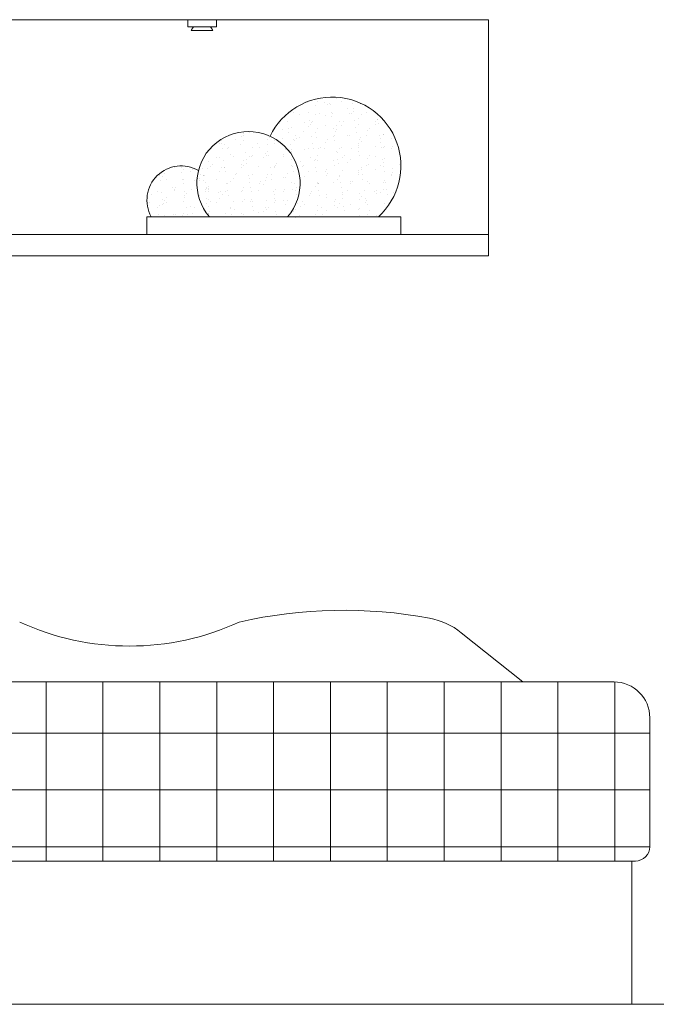
# Model space of a CAD drawing. Units: inches. Extents: x 1994 to 3075, y 3517 to 3950.
# Tile 28 of 58: x 1994.52987 to 1994.56485, y 3553.60329 to 3553.6574. Entities that reach past the tile are written whole.
import ezdxf

# ---------------------------------------------------------------- set-up
doc = ezdxf.new("R2010")
doc.units = ezdxf.units.IN
doc.layers.add('A-FURN-REFR', color=8, linetype='Continuous', lineweight=13)

msp = doc.modelspace()

# ---------------------------------------------------------------- linework, layer by layer
at = {"layer": 'A-FURN-REFR'}
for p, q in [((1994.492639873162, 3553.657398571457), (1994.555631999147, 3553.657398571457)), ((1994.539096566076, 3553.657004870669), (1994.539096566076, 3553.657398571457)), ((1994.539096566076, 3553.657398571457), (1994.540671369225, 3553.657398571457)), ((1994.540671369225, 3553.657004870669), (1994.540671369225, 3553.657398571457)), ((1994.555631999147, 3553.657398571457), (1994.555631999146, 3553.644427213402)), ((1994.539096566075, 3553.657004870669), (1994.540671369225, 3553.657004870669)), ((1994.539293416469, 3553.656808020276), (1994.540474518832, 3553.656808020276)), ((1994.545671567704, 3553.652825872638), (1994.545671567704, 3553.652825872638)), ((1994.546225091408, 3553.652899882358), (1994.546225091408, 3553.652899882358)), ((1994.546596443113, 3553.65285610945), (1994.546596443113, 3553.65285610945)), ((1994.546863187477, 3553.65281113167), (1994.546863187477, 3553.65281113167)), ((1994.547298108168, 3553.653085129387), (1994.547298108168, 3553.653085129387)), ((1994.547521318522, 3553.652886346262), (1994.547521318522, 3553.652886346262)), ((1994.544638888571, 3553.652286427241), (1994.544638888571, 3553.652286427241)), ((1994.544894170837, 3553.652309807435), (1994.544894170837, 3553.652309807435)), ((1994.545023122743, 3553.652512221382), (1994.545023122743, 3553.652512221382)), ((1994.545747841848, 3553.652271457508), (1994.545747841848, 3553.652271457508)), ((1994.546096139502, 3553.652697468411), (1994.546096139502, 3553.652697468411)), ((1994.546782116653, 3553.65272265839), (1994.546782116653, 3553.65272265839)), ((1994.546932370226, 3553.652714015634), (1994.546932370226, 3553.652714015634)), ((1994.546983745335, 3553.652323782936), (1994.546983745335, 3553.652323782936)), ((1994.547894002875, 3553.652521444812), (1994.547894002875, 3553.652521444812)), ((1994.547996152437, 3553.652267530656), (1994.547996152437, 3553.652267530656)), ((1994.548104907986, 3553.65226353994), (1994.548104907986, 3553.65226353994)), ((1994.548168273713, 3553.652766341061), (1994.548168273713, 3553.652766341061)), ((1994.548185978811, 3553.652352013221), (1994.548185978811, 3553.652352013221)), ((1994.548201166313, 3553.652516496956), (1994.548201166313, 3553.652516496956)), ((1994.548568633105, 3553.652769607105), (1994.548568633105, 3553.652769607105)), ((1994.548921027846, 3553.652297767468), (1994.548921027846, 3553.652297767468)), ((1994.544120035292, 3553.651720198246), (1994.544120035292, 3553.651720198246)), ((1994.544557817746, 3553.65219795396), (1994.544557817746, 3553.65219795396)), ((1994.544563313471, 3553.651828899384), (1994.544563313471, 3553.651828899384)), ((1994.54522152621, 3553.65217682022), (1994.54522152621, 3553.65217682022)), ((1994.545490065544, 3553.65174612286), (1994.545490065544, 3553.65174612286)), ((1994.545799216958, 3553.651881224811), (1994.545799216958, 3553.651881224811)), ((1994.54588060908, 3553.651738835511), (1994.54588060908, 3553.651738835511)), ((1994.545961679904, 3553.651827308792), (1994.545961679904, 3553.651827308792)), ((1994.546146401619, 3553.652207057032), (1994.546146401619, 3553.652207057032)), ((1994.546344334198, 3553.652244902675), (1994.546344334198, 3553.652244902675)), ((1994.546692034209, 3553.652133783835), (1994.546692034209, 3553.652133783835)), ((1994.547016637936, 3553.652073938831), (1994.547016637936, 3553.652073938831)), ((1994.547071277028, 3553.652237293845), (1994.547071277028, 3553.652237293845)), ((1994.547429776013, 3553.651792754602), (1994.547429776013, 3553.651792754602)), ((1994.547667125532, 3553.651785784226), (1994.547667125532, 3553.651785784226)), ((1994.548287000338, 3553.651864522816), (1994.548287000338, 3553.651864522816)), ((1994.548502792772, 3553.651978001632), (1994.548502792772, 3553.651978001632)), ((1994.548631744678, 3553.652180415578), (1994.548631744678, 3553.652180415578)), ((1994.54942769932, 3553.651804421491), (1994.54942769932, 3553.651804421491)), ((1994.549508770145, 3553.651892894772), (1994.549508770145, 3553.651892894772)), ((1994.549522903825, 3553.651916848242), (1994.549522903825, 3553.651916848242)), ((1994.542470918336, 3553.651200992831), (1994.542470918336, 3553.651200992831)), ((1994.544288096879, 3553.651358461884), (1994.544288096879, 3553.651358461884)), ((1994.544614688581, 3553.651438666687), (1994.544614688581, 3553.651438666687)), ((1994.544647581181, 3553.651188822582), (1994.544647581181, 3553.651188822582)), ((1994.544793400127, 3553.651499207083), (1994.544793400127, 3553.651499207083)), ((1994.545442826625, 3553.651261079797), (1994.545442826625, 3553.651261079797)), ((1994.545718275536, 3553.651529443895), (1994.545718275536, 3553.651529443895)), ((1994.545832109558, 3553.651631380706), (1994.545832109558, 3553.651631380706)), ((1994.546098855442, 3553.65120267968), (1994.546098855442, 3553.65120267968)), ((1994.546227807348, 3553.651405093626), (1994.546227807348, 3553.651405093626)), ((1994.546643150945, 3553.651559680707), (1994.546643150945, 3553.651559680707)), ((1994.54710247196, 3553.651421964691), (1994.54710247196, 3553.651421964691)), ((1994.547203400413, 3553.651279717062), (1994.547203400413, 3553.651279717062)), ((1994.547284471238, 3553.651368190343), (1994.547284471238, 3553.651368190343)), ((1994.547300824107, 3553.651590340655), (1994.547300824107, 3553.651590340655)), ((1994.547568026354, 3553.651589917519), (1994.547568026354, 3553.651589917519)), ((1994.548338375447, 3553.651474290118), (1994.548338375447, 3553.651474290118)), ((1994.548371268047, 3553.651224446013), (1994.548371268047, 3553.651224446013)), ((1994.548492901763, 3553.65162015433), (1994.548492901763, 3553.65162015433)), ((1994.548989916865, 3553.651326665777), (1994.548989916865, 3553.651326665777)), ((1994.54909868748, 3553.651414317057), (1994.54909868748, 3553.651414317057)), ((1994.549417777172, 3553.651650391142), (1994.549417777172, 3553.651650391142)), ((1994.549555796425, 3553.651667004138), (1994.549555796425, 3553.651667004138)), ((1994.540976954478, 3553.650774880818), (1994.540976954478, 3553.650774880818)), ((1994.541741367432, 3553.650819762049), (1994.541741367432, 3553.650819762049)), ((1994.542049971238, 3553.650960127848), (1994.542049971238, 3553.650960127848)), ((1994.542152382975, 3553.651015315854), (1994.542152382975, 3553.651015315854)), ((1994.542178923144, 3553.651162541795), (1994.542178923144, 3553.651162541795)), ((1994.542185275575, 3553.650765471749), (1994.542185275575, 3553.650765471749)), ((1994.54350194122, 3553.650838399314), (1994.54350194122, 3553.650838399314)), ((1994.543583012045, 3553.650926872594), (1994.543583012045, 3553.650926872594)), ((1994.54384783461, 3553.650784104248), (1994.54384783461, 3553.650784104248)), ((1994.544312677056, 3553.650890139674), (1994.544312677056, 3553.650890139674)), ((1994.544896886777, 3553.650815018703), (1994.544896886777, 3553.650815018703)), ((1994.544979101507, 3553.650755012633), (1994.544979101507, 3553.650755012633)), ((1994.545025838682, 3553.65101743265), (1994.545025838682, 3553.65101743265)), ((1994.545060172331, 3553.650843485914), (1994.545060172331, 3553.650843485914)), ((1994.545237552465, 3553.650920376486), (1994.545237552465, 3553.650920376486)), ((1994.545917943582, 3553.650979406566), (1994.545917943582, 3553.650979406566)), ((1994.546162427874, 3553.650950613298), (1994.546162427874, 3553.650950613298)), ((1994.546694750149, 3553.650638995105), (1994.546694750149, 3553.650638995105)), ((1994.546765617959, 3553.650801961348), (1994.546765617959, 3553.650801961348)), ((1994.547087303283, 3553.65098085011), (1994.547087303283, 3553.65098085011)), ((1994.547153847069, 3553.651031731993), (1994.547153847069, 3553.651031731993)), ((1994.547186739669, 3553.650781887887), (1994.547186739669, 3553.650781887887)), ((1994.547896718814, 3553.65102665608), (1994.547896718814, 3553.65102665608)), ((1994.548012178693, 3553.651011086922), (1994.548012178693, 3553.651011086922)), ((1994.548526191747, 3553.650820598612), (1994.548526191747, 3553.650820598612)), ((1994.548607262571, 3553.650909071893), (1994.548607262571, 3553.650909071893)), ((1994.548634460619, 3553.650685626847), (1994.548634460619, 3553.650685626847)), ((1994.548937054102, 3553.651041323733), (1994.548937054102, 3553.651041323733)), ((1994.549641630449, 3553.651015029997), (1994.549641630449, 3553.651015029997)), ((1994.549707477378, 3553.650870873877), (1994.549707477378, 3553.650870873877)), ((1994.549836429284, 3553.651073287823), (1994.549836429284, 3553.651073287823)), ((1994.549861929511, 3553.651071560545), (1994.549861929511, 3553.651071560545)), ((1994.550312708199, 3553.650867547327), (1994.550312708199, 3553.650867547327)), ((1994.540848002572, 3553.650572466871), (1994.540848002572, 3553.650572466871)), ((1994.540967854597, 3553.650572757729), (1994.540967854597, 3553.650572757729)), ((1994.541000747197, 3553.650322913624), (1994.541000747197, 3553.650322913624)), ((1994.541096001432, 3553.650521703602), (1994.541096001432, 3553.650521703602)), ((1994.541277642314, 3553.650313694884), (1994.541277642314, 3553.650313694884)), ((1994.541358713139, 3553.650402168165), (1994.541358713139, 3553.650402168165)), ((1994.542020876841, 3553.650551940413), (1994.542020876841, 3553.650551940413)), ((1994.542271109599, 3553.650113497608), (1994.542271109599, 3553.650113497608)), ((1994.542645865945, 3553.650396443273), (1994.542645865945, 3553.650396443273)), ((1994.54294575225, 3553.650582177225), (1994.54294575225, 3553.650582177225)), ((1994.543064158765, 3553.6503606436), (1994.543064158765, 3553.6503606436)), ((1994.543455637977, 3553.650556055733), (1994.543455637977, 3553.650556055733)), ((1994.543507013086, 3553.650165823036), (1994.543507013086, 3553.650165823036)), ((1994.543870627659, 3553.650612414037), (1994.543870627659, 3553.650612414037)), ((1994.544456624509, 3553.650240661069), (1994.544456624509, 3553.650240661069)), ((1994.544733415205, 3553.650536848441), (1994.544733415205, 3553.650536848441)), ((1994.544784790315, 3553.650146615743), (1994.544784790315, 3553.650146615743)), ((1994.544787510971, 3553.650271324068), (1994.544787510971, 3553.650271324068)), ((1994.545492781483, 3553.650251334128), (1994.545492781483, 3553.650251334128)), ((1994.54571238638, 3553.65030156088), (1994.54571238638, 3553.65030156088)), ((1994.545969318692, 3553.650589173868), (1994.545969318692, 3553.650589173868)), ((1994.546002211292, 3553.650339329763), (1994.546002211292, 3553.650339329763)), ((1994.54630189284, 3553.650295894184), (1994.54630189284, 3553.650295894184)), ((1994.546382963665, 3553.650384367465), (1994.546382963665, 3553.650384367465)), ((1994.546637261789, 3553.650331797692), (1994.546637261789, 3553.650331797692)), ((1994.547272573694, 3553.650129913747), (1994.547272573694, 3553.650129913747)), ((1994.547303540047, 3553.650095551924), (1994.547303540047, 3553.650095551924)), ((1994.547432491953, 3553.650297965871), (1994.547432491953, 3553.650297965871)), ((1994.547562137198, 3553.650362034504), (1994.547562137198, 3553.650362034504)), ((1994.548088409292, 3553.650342842899), (1994.548088409292, 3553.650342842899)), ((1994.548457102071, 3553.650572471872), (1994.548457102071, 3553.650572471872)), ((1994.548487012608, 3553.650392271316), (1994.548487012608, 3553.650392271316)), ((1994.548505508712, 3553.650483212901), (1994.548505508712, 3553.650483212901)), ((1994.548508477181, 3553.650182239174), (1994.548508477181, 3553.650182239174)), ((1994.549411888016, 3553.650422508127), (1994.549411888016, 3553.650422508127)), ((1994.549693005558, 3553.650624797299), (1994.549693005558, 3553.650624797299)), ((1994.549725898159, 3553.650374953194), (1994.549725898159, 3553.650374953194)), ((1994.54984898308, 3553.650361480163), (1994.54984898308, 3553.650361480163)), ((1994.549930053905, 3553.650449953444), (1994.549930053905, 3553.650449953444)), ((1994.550303372085, 3553.650307189301), (1994.550303372085, 3553.650307189301)), ((1994.550336763426, 3553.650452744939), (1994.550336763426, 3553.650452744939)), ((1994.540241928614, 3553.649621121321), (1994.540241928614, 3553.649621121321)), ((1994.540667875348, 3553.649844090464), (1994.540667875348, 3553.649844090464)), ((1994.540839859859, 3553.649835939171), (1994.540839859859, 3553.649835939171)), ((1994.541086581222, 3553.649670939484), (1994.541086581222, 3553.649670939484)), ((1994.541443897279, 3553.650008782297), (1994.541443897279, 3553.650008782297)), ((1994.541592750758, 3553.649874327276), (1994.541592750758, 3553.649874327276)), ((1994.542181639084, 3553.649667753064), (1994.542181639084, 3553.649667753064)), ((1994.542322484709, 3553.649723264911), (1994.542322484709, 3553.649723264911)), ((1994.542517626167, 3553.649904564088), (1994.542517626167, 3553.649904564088)), ((1994.542600433647, 3553.649854576435), (1994.542600433647, 3553.649854576435)), ((1994.542681504472, 3553.649943049716), (1994.542681504472, 3553.649943049716)), ((1994.543254655843, 3553.649853000092), (1994.543254655843, 3553.649853000092)), ((1994.543383607749, 3553.650055414039), (1994.543383607749, 3553.650055414039)), ((1994.543442501576, 3553.6499348009), (1994.543442501576, 3553.6499348009)), ((1994.543539905686, 3553.649915978931), (1994.543539905686, 3553.649915978931)), ((1994.544367376985, 3553.649965037712), (1994.544367376985, 3553.649965037712)), ((1994.544386950099, 3553.64990152515), (1994.544386950099, 3553.64990152515)), ((1994.544810268088, 3553.649706562914), (1994.544810268088, 3553.649706562914)), ((1994.545284260297, 3553.649623947742), (1994.545284260297, 3553.649623947742)), ((1994.545864110386, 3553.649818138469), (1994.545864110386, 3553.649818138469)), ((1994.546088045316, 3553.649687355623), (1994.546088045316, 3553.649687355623)), ((1994.546101571382, 3553.649707890949), (1994.546101571382, 3553.649707890949)), ((1994.546209135706, 3553.649654184555), (1994.546209135706, 3553.649654184555)), ((1994.546230523287, 3553.649910304895), (1994.546230523287, 3553.649910304895)), ((1994.547134011115, 3553.649684421367), (1994.547134011115, 3553.649684421367)), ((1994.547323948803, 3553.64973968105), (1994.547323948803, 3553.64973968105)), ((1994.547624684173, 3553.649836775735), (1994.547624684173, 3553.649836775735)), ((1994.547705754999, 3553.649925249015), (1994.547705754999, 3553.649925249015)), ((1994.548058886525, 3553.649714658178), (1994.548058886525, 3553.649714658178)), ((1994.548541369781, 3553.64993239507), (1994.548541369781, 3553.64993239507)), ((1994.548983761933, 3553.64974489499), (1994.548983761933, 3553.64974489499)), ((1994.54910140342, 3553.649919528325), (1994.54910140342, 3553.649919528325)), ((1994.549411200625, 3553.649883724449), (1994.549411200625, 3553.649883724449)), ((1994.549811732183, 3553.649722979054), (1994.549811732183, 3553.649722979054)), ((1994.549839145223, 3553.649578499092), (1994.549839145223, 3553.649578499092)), ((1994.549908637343, 3553.649775131802), (1994.549908637343, 3553.649775131802)), ((1994.538349954585, 3553.649268434922), (1994.538349954585, 3553.649268434922)), ((1994.53874159335, 3553.649274475566), (1994.53874159335, 3553.649274475566)), ((1994.538774485951, 3553.649024631461), (1994.538774485951, 3553.649024631461)), ((1994.538893768846, 3553.649147539603), (1994.538893768846, 3553.649147539603)), ((1994.539267433067, 3553.649068890523), (1994.539267433067, 3553.649068890523)), ((1994.539348503892, 3553.649157363803), (1994.539348503892, 3553.649157363803)), ((1994.539902052844, 3553.649228381359), (1994.539902052844, 3553.649228381359)), ((1994.540187152278, 3553.649235023055), (1994.540187152278, 3553.649235023055)), ((1994.540376134741, 3553.649329872007), (1994.540376134741, 3553.649329872007)), ((1994.540457205566, 3553.649418345287), (1994.540457205566, 3553.649418345287)), ((1994.540850718512, 3553.649077678141), (1994.540850718512, 3553.649077678141)), ((1994.540979670418, 3553.649280092088), (1994.540979670418, 3553.649280092088)), ((1994.541112027687, 3553.649265259867), (1994.541112027687, 3553.649265259867)), ((1994.541137956331, 3553.649280706786), (1994.541137956331, 3553.649280706786)), ((1994.541170848932, 3553.649030862681), (1994.541170848932, 3553.649030862681)), ((1994.542036903096, 3553.649295496679), (1994.542036903096, 3553.649295496679)), ((1994.542052687177, 3553.649465339117), (1994.542052687177, 3553.649465339117)), ((1994.542162651192, 3553.649376820721), (1994.542162651192, 3553.649376820721)), ((1994.542355377309, 3553.649473420806), (1994.542355377309, 3553.649473420806)), ((1994.542961778506, 3553.64932573349), (1994.542961778506, 3553.64932573349)), ((1994.543625739711, 3553.64926400479), (1994.543625739711, 3553.64926400479)), ((1994.54385055055, 3553.649289315518), (1994.54385055055, 3553.649289315518)), ((1994.543886653915, 3553.649355970303), (1994.543886653915, 3553.649355970303)), ((1994.543923224981, 3553.649395457986), (1994.543923224981, 3553.649395457986)), ((1994.544004295805, 3553.649483931267), (1994.544004295805, 3553.649483931267)), ((1994.544811529324, 3553.649386207115), (1994.544811529324, 3553.649386207115)), ((1994.544861643197, 3553.649316330217), (1994.544861643197, 3553.649316330217)), ((1994.544894535798, 3553.649066486112), (1994.544894535798, 3553.649066486112)), ((1994.545400385267, 3553.649312071306), (1994.545400385267, 3553.649312071306)), ((1994.545481456092, 3553.649400544586), (1994.545481456092, 3553.649400544586)), ((1994.545728412635, 3553.649045117146), (1994.545728412635, 3553.649045117146)), ((1994.546139420425, 3553.649297122924), (1994.546139420425, 3553.649297122924)), ((1994.546172313026, 3553.64904727882), (1994.546172313026, 3553.64904727882)), ((1994.546653288045, 3553.649075353957), (1994.546653288045, 3553.649075353957)), ((1994.546697466088, 3553.649144206373), (1994.546697466088, 3553.649144206373)), ((1994.547186901719, 3553.64935902002), (1994.547186901719, 3553.64935902002)), ((1994.547356841404, 3553.649489836944), (1994.547356841404, 3553.649489836944)), ((1994.547578163454, 3553.649105590769), (1994.547578163454, 3553.649105590769)), ((1994.547899434754, 3553.64953186735), (1994.547899434754, 3553.64953186735)), ((1994.548503038863, 3553.649135827581), (1994.548503038863, 3553.649135827581)), ((1994.548627203805, 3553.649280420928), (1994.548627203805, 3553.649280420928)), ((1994.548637176558, 3553.649190838116), (1994.548637176558, 3553.649190838116)), ((1994.548947475507, 3553.649377657285), (1994.548947475507, 3553.649377657285)), ((1994.549028546332, 3553.649466130565), (1994.549028546332, 3553.649466130565)), ((1994.549427914272, 3553.649166064393), (1994.549427914272, 3553.649166064393)), ((1994.549710193317, 3553.649376085144), (1994.549710193317, 3553.649376085144)), ((1994.549863107292, 3553.649332746356), (1994.549863107292, 3553.649332746356)), ((1994.549895999892, 3553.649082902251), (1994.549895999892, 3553.649082902251)), ((1994.550351337665, 3553.649007012116), (1994.550351337665, 3553.649007012116)), ((1994.550352789681, 3553.649196301205), (1994.550352789681, 3553.649196301205)), ((1994.550733991959, 3553.649424606), (1994.550733991959, 3553.649424606)), ((1994.537557064973, 3553.648831917442), (1994.537557064973, 3553.648831917442)), ((1994.537589957573, 3553.648582073337), (1994.537589957573, 3553.648582073337)), ((1994.537691800181, 3553.648759878627), (1994.537691800181, 3553.648759878627)), ((1994.537820752087, 3553.648962292573), (1994.537820752087, 3553.648962292573)), ((1994.537921828502, 3553.648590821784), (1994.537921828502, 3553.648590821784)), ((1994.538829650613, 3553.648591134808), (1994.538829650613, 3553.648591134808)), ((1994.538846703912, 3553.648621058596), (1994.538846703912, 3553.648621058596)), ((1994.539489663553, 3553.648583855028), (1994.539489663553, 3553.648583855028)), ((1994.539648749847, 3553.648690017165), (1994.539648749847, 3553.648690017165)), ((1994.539737110784, 3553.648585970638), (1994.539737110784, 3553.648585970638)), ((1994.53977157932, 3553.648651295408), (1994.53977157932, 3553.648651295408)), ((1994.539777701752, 3553.648892431112), (1994.539777701752, 3553.648892431112)), ((1994.539938352286, 3553.648852116292), (1994.539938352286, 3553.648852116292)), ((1994.539953427954, 3553.648838148661), (1994.539953427954, 3553.648838148661)), ((1994.539986320554, 3553.648588304556), (1994.539986320554, 3553.648588304556)), ((1994.540044848352, 3553.648815215446), (1994.540044848352, 3553.648815215446)), ((1994.540661986192, 3553.64861620745), (1994.540661986192, 3553.64861620745)), ((1994.541446613219, 3553.648513993566), (1994.541446613219, 3553.648513993566)), ((1994.541586861602, 3553.648646444262), (1994.541586861602, 3553.648646444262)), ((1994.541698926074, 3553.648870753558), (1994.541698926074, 3553.648870753558)), ((1994.541779996899, 3553.648959226837), (1994.541779996899, 3553.648959226837)), ((1994.542441211333, 3553.648821446664), (1994.542441211333, 3553.648821446664)), ((1994.542511737011, 3553.648676681073), (1994.542511737011, 3553.648676681073)), ((1994.542648581884, 3553.648901654541), (1994.542648581884, 3553.648901654541)), ((1994.543102788233, 3553.648500108388), (1994.543102788233, 3553.648500108388)), ((1994.543386323688, 3553.648560625308), (1994.543386323688, 3553.648560625308)), ((1994.54343661242, 3553.648706917885), (1994.54343661242, 3553.648706917885)), ((1994.543485442526, 3553.648917702272), (1994.543485442526, 3553.648917702272)), ((1994.54367711482, 3553.648873772092), (1994.54367711482, 3553.648873772092)), ((1994.54371000742, 3553.648623927987), (1994.54371000742, 3553.648623927987)), ((1994.544361487829, 3553.648737154698), (1994.544361487829, 3553.648737154698)), ((1994.544459340448, 3553.648745872337), (1994.544459340448, 3553.648745872337)), ((1994.544588292354, 3553.648948286284), (1994.544588292354, 3553.648948286284)), ((1994.545495497423, 3553.648756545398), (1994.545495497423, 3553.648756545398)), ((1994.5467231766, 3553.648852952856), (1994.5467231766, 3553.648852952856)), ((1994.546804247425, 3553.648941426137), (1994.546804247425, 3553.648941426137)), ((1994.547306255986, 3553.648600763193), (1994.547306255986, 3553.648600763193)), ((1994.547435207893, 3553.64880317714), (1994.547435207893, 3553.64880317714)), ((1994.547442675427, 3553.648837862804), (1994.547442675427, 3553.648837862804)), ((1994.548052997368, 3553.648486775164), (1994.548052997368, 3553.648486775164)), ((1994.548127038759, 3553.648482307687), (1994.548127038759, 3553.648482307687)), ((1994.548508224652, 3553.648988424169), (1994.548508224652, 3553.648988424169)), ((1994.548509693052, 3553.648899901571), (1994.548509693052, 3553.648899901571)), ((1994.548678578915, 3553.648890188231), (1994.548678578915, 3553.648890188231)), ((1994.548711471515, 3553.648640344126), (1994.548711471515, 3553.648640344126)), ((1994.548977872777, 3553.648517011976), (1994.548977872777, 3553.648517011976)), ((1994.549902748187, 3553.648547248787), (1994.549902748187, 3553.648547248787)), ((1994.55027026684, 3553.648918538836), (1994.55027026684, 3553.648918538836)), ((1994.550306088024, 3553.648812400569), (1994.550306088024, 3553.648812400569)), ((1994.537441105432, 3553.647981754375), (1994.537441105432, 3553.647981754375)), ((1994.537675791597, 3553.647930099196), (1994.537675791597, 3553.647930099196)), ((1994.538287694888, 3553.648196194052), (1994.538287694888, 3553.648196194052)), ((1994.538365925494, 3553.648085067644), (1994.538365925494, 3553.648085067644)), ((1994.538365980841, 3553.648011991187), (1994.538365980841, 3553.648011991187)), ((1994.538446996319, 3553.648173540925), (1994.538446996319, 3553.648173540925)), ((1994.538860319974, 3553.64837265732), (1994.538860319974, 3553.64837265732)), ((1994.538911695084, 3553.647982424623), (1994.538911695084, 3553.647982424623)), ((1994.53929085625, 3553.648042227999), (1994.53929085625, 3553.648042227999)), ((1994.540072154578, 3553.647936330416), (1994.540072154578, 3553.647936330416)), ((1994.540096223462, 3553.648424982748), (1994.540096223462, 3553.648424982748)), ((1994.540098453451, 3553.648040411848), (1994.540098453451, 3553.648040411848)), ((1994.540129116062, 3553.648175138643), (1994.540129116062, 3553.648175138643)), ((1994.540152441946, 3553.648132016359), (1994.540152441946, 3553.648132016359)), ((1994.540215731659, 3553.648072464811), (1994.540215731659, 3553.648072464811)), ((1994.540227405357, 3553.648242825795), (1994.540227405357, 3553.648242825795)), ((1994.54023386011, 3553.647938594312), (1994.54023386011, 3553.647938594312)), ((1994.540244644554, 3553.64812633259), (1994.540244644554, 3553.64812633259)), ((1994.540878489326, 3553.647975403959), (1994.540878489326, 3553.647975403959)), ((1994.541158735519, 3553.647968831124), (1994.541158735519, 3553.647968831124)), ((1994.541256682955, 3553.64837888854), (1994.541256682955, 3553.64837888854)), ((1994.54126114362, 3553.648392997843), (1994.54126114362, 3553.648392997843)), ((1994.541308058065, 3553.647988655843), (1994.541308058065, 3553.647988655843)), ((1994.542055403117, 3553.647970550385), (1994.542055403117, 3553.647970550385)), ((1994.542083610928, 3553.647999067936), (1994.542083610928, 3553.647999067936)), ((1994.542184355023, 3553.648172964332), (1994.542184355023, 3553.648172964332)), ((1994.542492586442, 3553.648431213968), (1994.542492586442, 3553.648431213968)), ((1994.542525479043, 3553.648181369862), (1994.542525479043, 3553.648181369862)), ((1994.542583934953, 3553.647933879393), (1994.542583934953, 3553.647933879393)), ((1994.543008486337, 3553.648029304748), (1994.543008486337, 3553.648029304748)), ((1994.543021717408, 3553.648411635108), (1994.543021717408, 3553.648411635108)), ((1994.543257371782, 3553.648358211361), (1994.543257371782, 3553.648358211361)), ((1994.543795841444, 3553.647971953846), (1994.543795841444, 3553.647971953846)), ((1994.543933361746, 3553.64805954156), (1994.543933361746, 3553.64805954156)), ((1994.544344508742, 3553.647952516659), (1994.544344508742, 3553.647952516659)), ((1994.544425579566, 3553.648040989939), (1994.544425579566, 3553.648040989939)), ((1994.544808233859, 3553.648458583822), (1994.544808233859, 3553.648458583822)), ((1994.544858237155, 3553.648089778371), (1994.544858237155, 3553.648089778371)), ((1994.544980369822, 3553.648414511971), (1994.544980369822, 3553.648414511971)), ((1994.545031744931, 3553.648024279274), (1994.545031744931, 3553.648024279274)), ((1994.545055235155, 3553.648182187763), (1994.545055235155, 3553.648182187763)), ((1994.545278371141, 3553.648396064728), (1994.545278371141, 3553.648396064728)), ((1994.545902739853, 3553.647957603259), (1994.545902739853, 3553.647957603259)), ((1994.546104287321, 3553.648213102217), (1994.546104287321, 3553.648213102217)), ((1994.54620324655, 3553.648426301541), (1994.54620324655, 3553.648426301541)), ((1994.546233239227, 3553.648415516164), (1994.546233239227, 3553.648415516164)), ((1994.54625814705, 3553.648395304679), (1994.54625814705, 3553.648395304679)), ((1994.546285394146, 3553.648375197142), (1994.546285394146, 3553.648375197142)), ((1994.546309522159, 3553.648005071981), (1994.546309522159, 3553.648005071981)), ((1994.547128121959, 3553.648456538352), (1994.547128121959, 3553.648456538352)), ((1994.547494050537, 3553.648447630106), (1994.547494050537, 3553.648447630106)), ((1994.547526943137, 3553.648197786002), (1994.547526943137, 3553.648197786002)), ((1994.547902150694, 3553.648037078618), (1994.547902150694, 3553.648037078618)), ((1994.548045967934, 3553.648393834407), (1994.548045967934, 3553.648393834407)), ((1994.548797305539, 3553.647988369985), (1994.548797305539, 3553.647988369985)), ((1994.549104119359, 3553.648424739594), (1994.549104119359, 3553.648424739594)), ((1994.549368759267, 3553.647934715958), (1994.549368759267, 3553.647934715958)), ((1994.549449830092, 3553.648023189238), (1994.549449830092, 3553.648023189238)), ((1994.549832484386, 3553.648440783122), (1994.549832484386, 3553.648440783122)), ((1994.549841861163, 3553.64808371036), (1994.549841861163, 3553.64808371036)), ((1994.549981833916, 3553.64843092811), (1994.549981833916, 3553.64843092811)), ((1994.550033209026, 3553.648040695413), (1994.550033209026, 3553.648040695413)), ((1994.537085726223, 3553.647808533077), (1994.537085726223, 3553.647808533077)), ((1994.537727166706, 3553.647539866498), (1994.537727166706, 3553.647539866498)), ((1994.537823468026, 3553.647467503843), (1994.537823468026, 3553.647467503843)), ((1994.537928143039, 3553.64760731193), (1994.537928143039, 3553.64760731193)), ((1994.538840814755, 3553.647393175582), (1994.538840814755, 3553.647393175582)), ((1994.538896484786, 3553.647652750872), (1994.538896484786, 3553.647652750872)), ((1994.538944587684, 3553.647732580518), (1994.538944587684, 3553.647732580518)), ((1994.539025436692, 3553.647855164819), (1994.539025436692, 3553.647855164819)), ((1994.539688716827, 3553.647625949195), (1994.539688716827, 3553.647625949195)), ((1994.539765690165, 3553.647423412394), (1994.539765690165, 3553.647423412394)), ((1994.539769787652, 3553.647714422476), (1994.539769787652, 3553.647714422476)), ((1994.540123529687, 3553.647546097718), (1994.540123529687, 3553.647546097718)), ((1994.540214950086, 3553.647523164502), (1994.540214950086, 3553.647523164502)), ((1994.540359636047, 3553.647409174965), (1994.540359636047, 3553.647409174965)), ((1994.540797418501, 3553.647886930679), (1994.540797418501, 3553.647886930679)), ((1994.540853434452, 3553.64758288941), (1994.540853434452, 3553.64758288941)), ((1994.540982386357, 3553.647785303356), (1994.540982386357, 3553.647785303356)), ((1994.541340950665, 3553.647738811738), (1994.541340950665, 3553.647738811738)), ((1994.541602887857, 3553.647390000527), (1994.541602887857, 3553.647390000527)), ((1994.542120209835, 3553.64742781223), (1994.542120209835, 3553.64742781223)), ((1994.54220128066, 3553.64751628551), (1994.54220128066, 3553.64751628551)), ((1994.542527763266, 3553.647420237339), (1994.542527763266, 3553.647420237339)), ((1994.542611313067, 3553.647529395722), (1994.542611313067, 3553.647529395722)), ((1994.542651297824, 3553.64740686581), (1994.542651297824, 3553.64740686581)), ((1994.543452638676, 3553.647450474151), (1994.543452638676, 3553.647450474151)), ((1994.543847216554, 3553.647581721149), (1994.543847216554, 3553.647581721149)), ((1994.54385326649, 3553.647794526786), (1994.54385326649, 3553.647794526786)), ((1994.543906726287, 3553.647474760944), (1994.543906726287, 3553.647474760944)), ((1994.544377514085, 3553.647480710963), (1994.544377514085, 3553.647480710963)), ((1994.544591008293, 3553.647453497553), (1994.544591008293, 3553.647453497553)), ((1994.545064637532, 3553.647774435169), (1994.545064637532, 3553.647774435169)), ((1994.545383886573, 3553.647391374263), (1994.545383886573, 3553.647391374263)), ((1994.545775120467, 3553.647748688403), (1994.545775120467, 3553.647748688403)), ((1994.545821669028, 3553.647869129978), (1994.545821669028, 3553.647869129978)), ((1994.54634241476, 3553.647755227876), (1994.54634241476, 3553.647755227876)), ((1994.546699995876, 3553.647778925215), (1994.546699995876, 3553.647778925215)), ((1994.546700182028, 3553.647649417643), (1994.546700182028, 3553.647649417643)), ((1994.547144460361, 3553.647410011528), (1994.547144460361, 3553.647410011528)), ((1994.547225531186, 3553.647498484809), (1994.547225531186, 3553.647498484809)), ((1994.547608185479, 3553.647916078693), (1994.547608185479, 3553.647916078693)), ((1994.547612777161, 3553.64754581186), (1994.547612777161, 3553.64754581186)), ((1994.547624871285, 3553.647809162026), (1994.547624871285, 3553.647809162026)), ((1994.548510940591, 3553.647493635438), (1994.548510940591, 3553.647493635438)), ((1994.548549746695, 3553.647839398838), (1994.548549746695, 3553.647839398838)), ((1994.548639892497, 3553.647696049385), (1994.548639892497, 3553.647696049385)), ((1994.548848680648, 3553.647598137287), (1994.548848680648, 3553.647598137287)), ((1994.548930976813, 3553.647456960244), (1994.548930976813, 3553.647456960244)), ((1994.549474622104, 3553.64786963565), (1994.549474622104, 3553.64786963565)), ((1994.549712909257, 3553.647881296414), (1994.549712909257, 3553.647881296414)), ((1994.550066101626, 3553.647790851308), (1994.550066101626, 3553.647790851308)), ((1994.550399497513, 3553.647899872462), (1994.550399497513, 3553.647899872462)), ((1994.536991063937, 3553.647332701958), (1994.536991063937, 3553.647332701958)), ((1994.537464417921, 3553.647101244767), (1994.537464417921, 3553.647101244767)), ((1994.537545488746, 3553.647189718046), (1994.537545488746, 3553.647189718046)), ((1994.53769451612, 3553.647265089896), (1994.53769451612, 3553.647265089896)), ((1994.537760059307, 3553.647290022393), (1994.537760059307, 3553.647290022393)), ((1994.537915939346, 3553.64736293877), (1994.537915939346, 3553.64736293877)), ((1994.539030421708, 3553.647080606377), (1994.539030421708, 3553.647080606377)), ((1994.539250934373, 3553.64714819348), (1994.539250934373, 3553.64714819348)), ((1994.539492379493, 3553.647089066297), (1994.539492379493, 3553.647089066297)), ((1994.540156422288, 3553.647296253613), (1994.540156422288, 3553.647296253613)), ((1994.540266325195, 3553.647132931804), (1994.540266325195, 3553.647132931804)), ((1994.540299217796, 3553.646883087699), (1994.540299217796, 3553.646883087699)), ((1994.540678012448, 3553.647359763715), (1994.540678012448, 3553.647359763715)), ((1994.541426784689, 3553.647086837596), (1994.541426784689, 3553.647086837596)), ((1994.541449329158, 3553.647019204834), (1994.541449329158, 3553.647019204834)), ((1994.54168242738, 3553.646950056516), (1994.54168242738, 3553.646950056516)), ((1994.542662688176, 3553.647139163024), (1994.542662688176, 3553.647139163024)), ((1994.542695580776, 3553.646889318919), (1994.542695580776, 3553.646889318919)), ((1994.543260087722, 3553.64686342263), (1994.543260087722, 3553.64686342263)), ((1994.543389039628, 3553.647065836577), (1994.543389039628, 3553.647065836577)), ((1994.543443001168, 3553.646968693781), (1994.543443001168, 3553.646968693781)), ((1994.543524071993, 3553.647057167061), (1994.543524071993, 3553.647057167061)), ((1994.543880109154, 3553.647331877044), (1994.543880109154, 3553.647331877044)), ((1994.544462056387, 3553.647251083607), (1994.544462056387, 3553.647251083607)), ((1994.544920161455, 3553.6468853071), (1994.544920161455, 3553.6468853071)), ((1994.545001232279, 3553.64697378038), (1994.545001232279, 3553.64697378038)), ((1994.545157886382, 3553.647312669751), (1994.545157886382, 3553.647312669751)), ((1994.545294397397, 3553.647139620994), (1994.545294397397, 3553.647139620994)), ((1994.545498213362, 3553.647261756666), (1994.545498213362, 3553.647261756666)), ((1994.546219272806, 3553.647169857806), (1994.546219272806, 3553.647169857806)), ((1994.546235955167, 3553.646920727433), (1994.546235955167, 3553.646920727433)), ((1994.546428248783, 3553.647103253735), (1994.546428248783, 3553.647103253735)), ((1994.546706677907, 3553.646932255814), (1994.546706677907, 3553.646932255814)), ((1994.547144148215, 3553.647200094618), (1994.547144148215, 3553.647200094618)), ((1994.547308971926, 3553.647105974462), (1994.547308971926, 3553.647105974462)), ((1994.547437923832, 3553.647308388409), (1994.547437923832, 3553.647308388409)), ((1994.54766415227, 3553.647155579163), (1994.54766415227, 3553.647155579163)), ((1994.547697044871, 3553.646905735058), (1994.547697044871, 3553.646905735058)), ((1994.548069023624, 3553.647230331429), (1994.548069023624, 3553.647230331429)), ((1994.548467251695, 3553.646950893079), (1994.548467251695, 3553.646950893079)), ((1994.548548322519, 3553.64703936636), (1994.548548322519, 3553.64703936636)), ((1994.548881573249, 3553.647348293182), (1994.548881573249, 3553.647348293182)), ((1994.548993899033, 3553.647260568241), (1994.548993899033, 3553.647260568241)), ((1994.549106835298, 3553.646929950863), (1994.549106835298, 3553.646929950863)), ((1994.549918774442, 3553.647290805053), (1994.549918774442, 3553.647290805053)), ((1994.536857346972, 3553.646571799804), (1994.550814563623, 3553.646571799804)), ((1994.536857346972, 3553.646571799804), (1994.536857346972, 3553.645587547835)), ((1994.537487813263, 3553.646685325632), (1994.537487813263, 3553.646685325632)), ((1994.537845893331, 3553.646638048252), (1994.537845893331, 3553.646638048252)), ((1994.538290410828, 3553.646701405321), (1994.538290410828, 3553.646701405321)), ((1994.538412688672, 3553.646715562444), (1994.538412688672, 3553.646715562444)), ((1994.538787209254, 3553.646642126317), (1994.538787209254, 3553.646642126317)), ((1994.538868280079, 3553.646730599597), (1994.538868280079, 3553.646730599597)), ((1994.539081796818, 3553.64669037368), (1994.539081796818, 3553.64669037368)), ((1994.539337564082, 3553.646745799257), (1994.539337564082, 3553.646745799257)), ((1994.540227970954, 3553.646710711298), (1994.540227970954, 3553.646710711298)), ((1994.540230121296, 3553.646748037063), (1994.540230121296, 3553.646748037063)), ((1994.540242256311, 3553.646644279472), (1994.540242256311, 3553.646644279472)), ((1994.540247360493, 3553.646631543858), (1994.540247360493, 3553.646631543858)), ((1994.540262439491, 3553.646776036068), (1994.540262439491, 3553.646776036068)), ((1994.541152846363, 3553.646740948109), (1994.541152846363, 3553.646740948109)), ((1994.541478159798, 3553.646696604899), (1994.541478159798, 3553.646696604899)), ((1994.542077721772, 3553.646771184921), (1994.542077721772, 3553.646771184921)), ((1994.542187070963, 3553.646678175601), (1994.542187070963, 3553.646678175601)), ((1994.543002597181, 3553.646801421733), (1994.543002597181, 3553.646801421733)), ((1994.54392747259, 3553.646831658545), (1994.54392747259, 3553.646831658545)), ((1994.543965943178, 3553.646679902903), (1994.543965943178, 3553.646679902903)), ((1994.545033986501, 3553.646533066457), (1994.545033986501, 3553.646533066457)), ((1994.545243720406, 3553.646660695611), (1994.545243720406, 3553.646660695611)), ((1994.546107003261, 3553.646718313486), (1994.546107003261, 3553.646718313486)), ((1994.546479623893, 3553.646713021038), (1994.546479623893, 3553.646713021038)), ((1994.54669410672, 3553.6465510422), (1994.54669410672, 3553.6465510422)), ((1994.547618982129, 3553.646581279012), (1994.547618982129, 3553.646581279012)), ((1994.548543857539, 3553.646611515824), (1994.548543857539, 3553.646611515824)), ((1994.548967407273, 3553.646696319042), (1994.548967407273, 3553.646696319042)), ((1994.549468732948, 3553.646641752636), (1994.549468732948, 3553.646641752636)), ((1994.550814563623, 3553.646571799804), (1994.550814563623, 3553.645587547835)), ((1994.492639873162, 3553.645587547835), (1994.555631999147, 3553.645587547835)), ((1994.492639873162, 3553.644427213402), (1994.555631999146, 3553.644427213402)), ((1994.557504748733, 3553.621010566067), (1994.554126580377, 3553.623713100752)), ((1994.485750109383, 3553.621010566067), (1994.562521762926, 3553.621010566067)), ((1994.531314222183, 3553.611168046383), (1994.531314222183, 3553.621010566067)), ((1994.534439222183, 3553.611168046383), (1994.534439222183, 3553.621010566067)), ((1994.537564222183, 3553.611168046383), (1994.537564222183, 3553.621010566067)), ((1994.540689222183, 3553.611168046383), (1994.540689222183, 3553.621010566067)), ((1994.543814222183, 3553.611168046383), (1994.543814222183, 3553.621010566067)), ((1994.546939222183, 3553.611168046383), (1994.546939222183, 3553.621010566067)), ((1994.550064222183, 3553.611168046383), (1994.550064222183, 3553.621010566067)), ((1994.553189222183, 3553.611168046383), (1994.553189222183, 3553.621010566067)), ((1994.556314222183, 3553.611168046383), (1994.556314222183, 3553.621010566067)), ((1994.559439222183, 3553.611168046383), (1994.559439222183, 3553.621010566067)), ((1994.562564222183, 3553.611168046383), (1994.562564222183, 3553.621010108106)), ((1994.564490266863, 3553.61904206213), (1994.564490266863, 3553.611955447957)), ((1994.483781605446, 3553.618198825726), (1994.564490266863, 3553.618198825726)), ((1994.483781605446, 3553.615073825726), (1994.564490266863, 3553.615073825726)), ((1994.483781633293, 3553.611948825726), (1994.564490239016, 3553.611948825726)), ((1994.48456900702, 3553.611168046383), (1994.563702865288, 3553.611168046383)), ((1994.563506014895, 3553.611168046383), (1994.563506014895, 3553.603294030634)), ((1994.602439621408, 3553.603294030634), (1994.442865031001, 3553.603294030634))]:
    msp.add_line(p, q, dxfattribs=at)
for centre, radius, start, end in [((1994.53988396765, 3553.656561957283), 0.0006397637796166, 136.1869385529525, 157.3801350610466), ((1994.53988396765, 3553.656561957283), 0.0006397637796166, 22.61986494091335, 43.81306144798317), ((1994.547035036064, 3553.649367075394), 0.0037795275590551, 312.3040659485178, 154.459902867195), ((1994.542438366796, 3553.648422193504), 0.0028346456692913, 319.2486367054326, 220.7513632947834), ((1994.538747110751, 3553.647477311614), 0.0018897637795276, 60.07893087766362, 208.6309898387077), ((1994.547662229048, 3553.599251933981), 0.0256956399605624, 79.39359087275909, 102.8851461685604), ((1994.535899082601, 3553.637411704167), 0.0144326341621686, 245.2905486962294, 294.7094513037706), ((1994.551667151056, 3553.620638814101), 0.0039370078740157, 51.34019174472132, 79.39359087275909), ((1994.562521762926, 3553.61904206213), 0.0019685039370079, 1.9853989e-09, 90), ((1994.563702865288, 3553.611955447957), 0.0007874015748031, 270, 6.617996e-10)]:
    msp.add_arc(centre, radius, start, end, dxfattribs=at)

doc.saveas('drawing.dxf')
